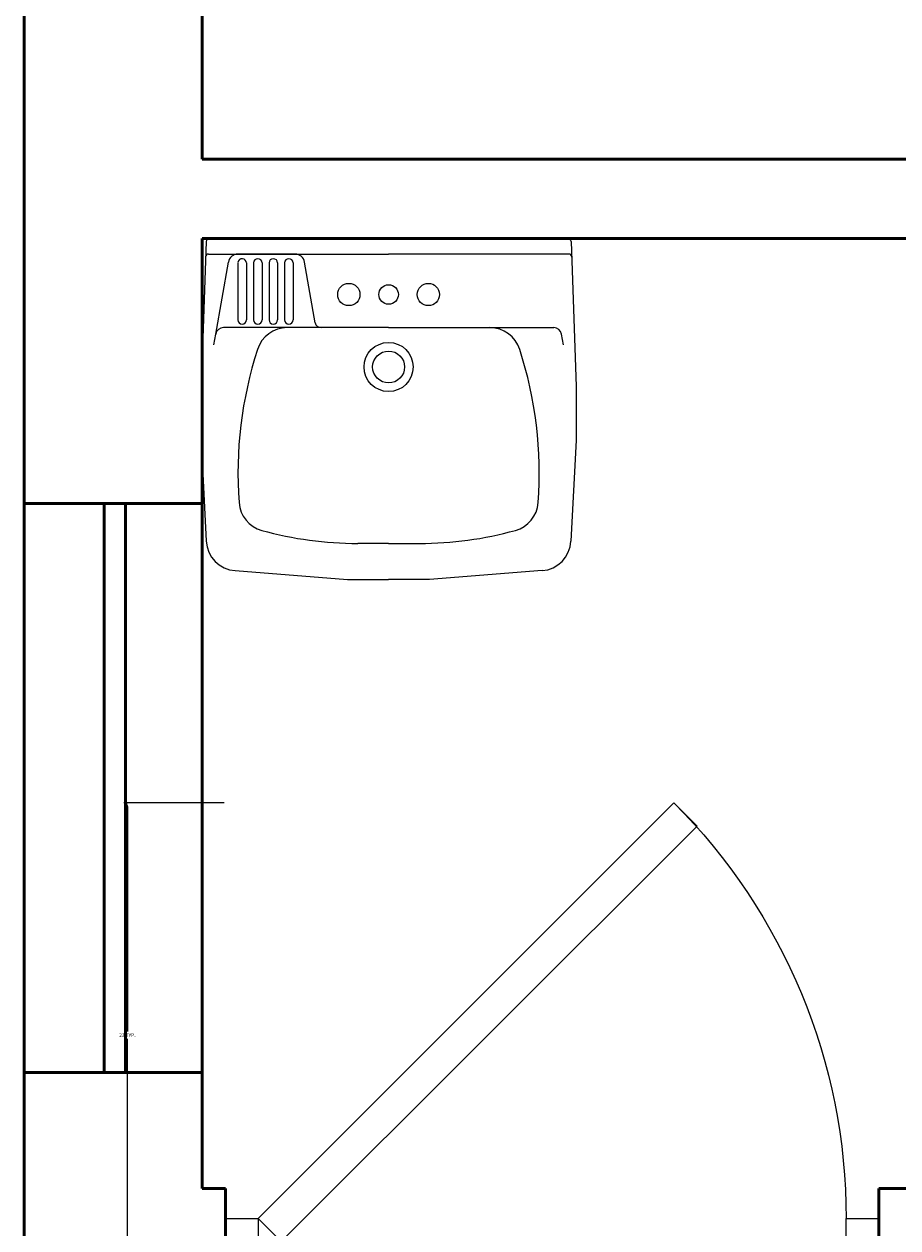
# Model space of a CAD drawing. Units: inches. Extents: x 64 to 1167, y 117 to 939.
# Tile 6 of 56: x 122 to 166, y 583 to 644. Entities that reach past the tile are written whole.
import ezdxf

# ---------------------------------------------------------------- set-up
doc = ezdxf.new("R2010")
doc.units = ezdxf.units.IN
doc.header["$MEASUREMENT"] = 0
for name, color, linetype, lineweight in [('A-ANNO-DIMS', 2, 'Continuous', 18), ('A-DOOR', 4, 'Continuous', 25), ('A-FLOR-FIXT', 8, 'Continuous', 18), ('A-WALL', 7, 'Continuous', 50)]:
    doc.layers.add(name, color=color, linetype=linetype, lineweight=lineweight)
doc.styles.get("Standard").update_dxf_attribs({"font": 'arial.ttf'})
doc.dimstyles.get("Standard").update_dxf_attribs({"dimtxt": 0.18, "dimasz": 0.18, "dimexe": 0.18, "dimexo": 0.0625, "dimgap": 0.09, "dimtad": 0, "dimtih": 1, "dimtoh": 1, "dimdec": 4, "dimzin": 0, "dimdsep": 46, "dimtxsty": 'Standard', "dimcen": 0.09, "dimadec": 0, "dimazin": 0, "dimtfac": 1, "dimtdec": 4, "dimtofl": 0, "dimtmove": 0, "dimatfit": 3, "dimfxl": 1, "dimtolj": 1, "dimtzin": 0, "dimarcsym": 0})

# ---------------------------------------------------------------- blocks, each defined once
blk = doc.blocks.new('A$C68901CC0')
for p, q in [((10.95466834153159, 26.61577842384394), (12.3466108238266, 28.00772090643226)), ((12.3466108238266, 28.00772090643226), (37.40157551217649, 2.952756218669026)), ((36.00963302988149, 1.560813736080697), (10.95466834153159, 26.61577842384394)), ((7.090268874e-07, 2.952756218669026), (7.090268874e-07, 3.131572157e-07)), ((1.968504646034761, 2.952756218669026), (7.090268874e-07, 2.952756218669026)), ((1.968504646034761, 3.131572157e-07), (1.968504646034761, 2.952756218669026)), ((37.40157551217649, 2.952756218669026), (36.00963302988149, 1.560813736080697)), ((37.40157551217649, 2.952756218669026), (37.40157551217649, 3.131572157e-07)), ((39.37007944918437, 2.952756218669026), (37.40157551217649, 2.952756218669026)), ((39.37007944918437, 3.131572157e-07), (39.37007944918437, 2.952756218669026)), ((7.090268874e-07, 3.131572157e-07), (1.968504646034761, 3.131572157e-07)), ((37.40157551217649, 3.131572157e-07), (39.37007944918437, 3.131572157e-07))]:
    blk.add_line(p, q)
blk.add_arc((37.40157551371189, 2.952756218643245), 35.43307086614174, 135.0000000005895, 180)
blk = doc.blocks.new('A$C056A4ABE')
at = {"ltscale": 20}
for p, q in [((0.0064960553054334, 0.4339203704876127), (-4.08590495e-08, 0.2478965153641184)), ((0.2406308635145251, 0.4377807724958985), (0.0104936186135092, 0.4377807724958985)), ((0.2406308635145251, 0.4377807724958985), (0.4707681084155411, 0.4377807724958985)), ((0.4747656717236169, 0.4339203704876127), (0.4812617678880998, 0.2478965153641184)), ((0.0097952032238027, 0.4177807724990999), (0.2406308635145251, 0.4177807724990999)), ((0.1204792184480539, 0.4177807724990999), (0.0474567092269354, 0.4177807724990999)), ((0.1099904730581329, 0.4177807724990999), (0.0579454546168563, 0.4177807724990999)), ((0.4714665238052476, 0.4177807724990999), (0.2406308635145251, 0.4177807724990999)), ((0.018847982942134, 0.3150172542736982), (0.0351466123147475, 0.4074513747182209)), ((0.0472450566530824, 0.4062810405885103), (0.0472450566530824, 0.3332810405845521)), ((0.0582450566535044, 0.4062810405885103), (0.0582450566535044, 0.3332810405845521)), ((0.067245056653519, 0.4062810405885103), (0.067245056653519, 0.3332810405845521)), ((0.0782450566530315, 0.4062810405885103), (0.0782450566530315, 0.3332810405845521)), ((0.0872450566530461, 0.4062810405885103), (0.0872450566530461, 0.3332810405845521)), ((0.0982450566534681, 0.4062810405885103), (0.0982450566534681, 0.3332810405845521)), ((0.1072450566534826, 0.4062810405885103), (0.1072450566534826, 0.3332810405845521)), ((0.1182450566529951, 0.4062810405885103), (0.1182450566529951, 0.3332810405845521)), ((0.1465380526005902, 0.3294784111640183), (0.1327893153602417, 0.4074513747182209)), ((0.0164258705844986, 0.3012807724953745), (0.018847982942134, 0.3150172542736982)), ((0.2406308635145251, 0.3232807724998565), (0.0286960604726119, 0.3232807724998565)), ((0.2406308635145251, 0.3232807724998565), (0.146816124464749, 0.3232807724998565)), ((0.2406308635145251, 0.3232807724998565), (0.3344456025633917, 0.3232807724998565)), ((0.2406308635145251, 0.3232807724998565), (0.4525656665564384, 0.3232807724998565)), ((0.4648358564436422, 0.3012807724953745), (0.4624137440869163, 0.3150172542736982)), ((-4.08590495e-08, 0.2478965153641184), (-4.08590495e-08, 0.1788965153682511)), ((0.4812617678880998, 0.2478965153641184), (0.4812617678880998, 0.1788965153682511)), ((-4.08590495e-08, 0.1788965153682511), (0.006799495849009, 0.0491536260233261)), ((0.4812617678880998, 0.1788965153682511), (0.4744622311791318, 0.0491536260233261)), ((0.2406308635145251, 0.0462807724979939), (0.2010764077012936, 0.0462807724979939)), ((0.2406308635145251, 0.0462807724979939), (0.2801853193268471, 0.0462807724979939)), ((0.0436063134102369, 0.0113703709212132), (0.1880805119926663, 4.8967195e-09)), ((0.1880805119926663, 4.8967195e-09), (0.2406308635145251, 4.8967195e-09)), ((0.2931812150354744, 4.8967195e-09), (0.2406308635145251, 4.8967195e-09)), ((0.4376554136188134, 0.0113703709212132), (0.2931812150354744, 4.8967195e-09))]:
    blk.add_line(p, q, dxfattribs=at)
for centre, radius in [((0.1896308635141395, 0.365780772495782), 0.01425), ((0.2406308635145251, 0.365780772495782), 0.0125), ((0.2916308635140012, 0.365780772495782), 0.01425), ((0.2406308635145251, 0.2727807725023013), 0.0315), ((0.2406308635145251, 0.2727807725023013), 0.0205)]:
    blk.add_circle(centre, radius, dxfattribs=at)
for centre, radius, start, end in [((0.0104936186135092, 0.4337807725023595), 0.004, 90, 178.0000000002043), ((0.4707681084155411, 0.4337807725023595), 0.004, 1.999999999795639, 90), ((0.0097952032238027, 0.413780772498285), 0.004, 90, 178.0000000002043), ((0.0474567092269354, 0.4052807725020103), 0.0125, 90, 169.9999999999448), ((0.1204792184480539, 0.4052807725020103), 0.0125, 10.00000000005521, 90), ((0.4714665238052476, 0.413780772498285), 0.004, 1.999999999795639, 90), ((0.0527450566532934, 0.4062810405885103), 0.0055, 0, 172.1464139600562), ((0.0727450566528205, 0.4062810405885103), 0.0055, 0, 180), ((0.0927450566532571, 0.4062810405885103), 0.0055, 0, 180), ((0.1127450566527841, 0.4062810405885103), 0.0055, 0, 180), ((0.0527450566532934, 0.3332810405845521), 0.0055, 180, 0), ((0.0727450566528205, 0.3332810405845521), 0.0055, 180, 0), ((0.0927450566532571, 0.3332810405845521), 0.0055, 180, 0), ((0.1127450566527841, 0.3332810405845521), 0.0055, 180, 0), ((0.1539241107484486, 0.3307807724995655), 0.0075, 190.0000000000552, 270), ((0.0286960604726119, 0.3132807724978193), 0.01, 90, 169.9999999999448), ((0.110630863514416, 0.2832807724989834), 0.04, 90, 162.5107076218657), ((0.3706308635146343, 0.2832807724989834), 0.04, 17.48929237813428, 90), ((0.4525656665564384, 0.3132807724978193), 0.01, 10.00000000005521, 90), ((0.5633260594686363, 0.1362824146417552), 0.5159623081565683, 162.0492268008092, 184.1816890620389), ((-0.082064332439586, 0.1362824146417552), 0.5159623081565683, 355.8183109379611, 17.95077319919074), ((0.0886308635144815, 0.1015752147432067), 0.04, 184.1812829145062, 254.5087296059769), ((0.3926308635145688, 0.1015752147432067), 0.04, 285.4912703940231, 355.8187170854937), ((0.2010764077012936, 0.5072807725009625), 0.4610000000000002, 254.5087296059769, 270), ((0.2801853193268471, 0.5072807725009625), 0.4610000000000002, 270, 285.4912703940231), ((0.0467446772390758, 0.0512470642715925), 0.04, 183.0000000000061, 265.4999999999645), ((0.434517049789065, 0.0512470642715925), 0.04, 274.5000000000355, 356.9999999999938)]:
    blk.add_arc(centre, radius, start, end, dxfattribs=at)
blk = doc.blocks.new('*D61')
at = {"layer": 'A-ANNO-DIMS', "color": 0, "lineweight": -2, "transparency": 16777216}
for p, q in [((132.2138083222863, 604.6754863829213), (127.1463797540431, 604.6754863829213)), ((127.3263797540431, 604.4954863829214), (127.3263797540431, 593.1195845991894)), ((127.3263797540431, 581.3797537567943), (127.3263797540431, 592.7556555405264)), ((132.2138083222863, 581.1997537567943), (127.1463797540431, 581.1997537567943))]:
    blk.add_line(p, q, dxfattribs=at)
for points in [[(127.2963797540431, 604.4954863829214), (127.3563797540431, 604.4954863829214), (127.3263797540431, 604.6754863829213)], [(127.2963797540431, 581.3797537567943), (127.3563797540431, 581.3797537567943), (127.3263797540431, 581.1997537567943)]]:
    blk.add_solid(points, dxfattribs=at)
at = {"layer": 'Defpoints', "color": 0, "lineweight": -2, "transparency": 16777216}
for p in [(127.3263797540431, 604.6754863829213), (132.2763083222863, 604.6754863829213), (132.2763083222863, 581.1997537567943)]:
    blk.add_point(p, dxfattribs=at)
at = {"layer": 'A-ANNO-DIMS', "color": 0, "transparency": 16777216, "insert": (127.3263797540433, 592.9376200698576), "char_height": 0.18, "attachment_point": 5}
blk.add_mtext('\\A1;23 TYP.', dxfattribs=at)

msp = doc.modelspace()

# ---------------------------------------------------------------- linework, layer by layer
at = {"layer": 'A-WALL'}
for p, q in [((122.1072888543381, 863.1997537567942), (122.1072888543381, 155.1997537567943)), ((131.1072888543381, 781.1997537567942), (131.1072888543381, 637.1997537567942)), ((245.6090488124727, 637.1997537567942), (131.1072888543381, 637.1997537567942)), ((131.1072888543381, 633.1997537567943), (131.1072888543381, 585.1997537567942)), ((245.6090488124727, 633.1997537567943), (131.1072888543381, 633.1997537567943)), ((122.1072888543381, 619.8116554420988), (131.1072888543381, 619.8116554420988)), ((126.155003042033, 619.8116554420988), (126.155003042033, 591.0487833032248)), ((127.2258843451341, 619.8116554420988), (127.2258843451341, 591.0487833032248)), ((122.107288854338, 591.0487833032248), (131.1072888543381, 591.0487833032248)), ((132.2763083222862, 585.1997537567942), (131.1072888543381, 585.1997537567942)), ((132.2763083222862, 585.1997537567942), (132.2763083222862, 581.1997537567942)), ((255.1072888543381, 585.1997537567942), (165.2758321105744, 585.1997537567942)), ((165.2758321105744, 585.1997537567942), (165.2758321105744, 581.1997537567942))]:
    msp.add_line(p, q, dxfattribs=at)

# ---------------------------------------------------------------- block references
at = {"layer": 'A-DOOR', "xscale": -0.8381879042225197, "yscale": 0.8381879042225197, "zscale": 0.8381879042225197}
msp.add_blockref('A$C68901CC0', (165.2758327048722, 581.1997534943096), dxfattribs=at)
at = {"layer": 'A-FLOR-FIXT', "xscale": 39.37007874015748, "yscale": 39.37007874015748, "zscale": 39.37007874015748}
msp.add_blockref('A$C056A4ABE', (131.0432115847088, 615.9642902727037), dxfattribs=at)

# ---------------------------------------------------------------- dimensions: what is measured, and where the dimension line sits
at = {"layer": 'A-ANNO-DIMS'}
dim = msp.add_linear_dim(base=(127.3263797540431, 604.6754863829213), p1=(132.2763083222862, 581.1997537567942), p2=(132.2763083222862, 604.6754863829212), angle=90, text='<> TYP.', dimstyle='Standard', override={"dimdec": 0, "dimlfac": 1, "dimrnd": 0, "dimzin": 0, "dimdsep": 46, "dimlunit": 2}, dxfattribs=at)
dim.commit()
dim.dimension.update_dxf_attribs({"geometry": '*D61', "text_midpoint": (127.3263797540433, 592.9376200698576)})

doc.saveas('drawing.dxf')
